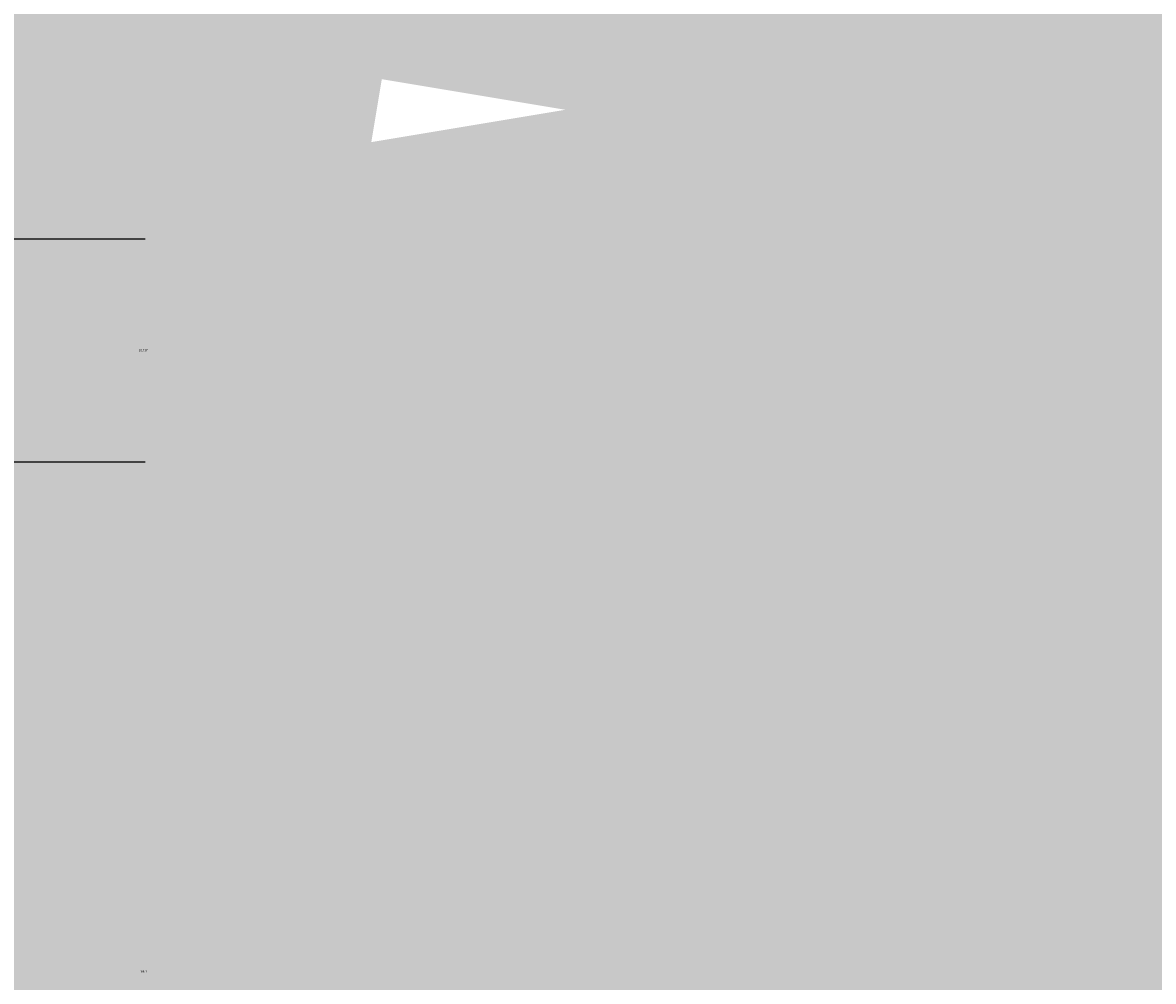
# Model space of a CAD drawing. Units: millimetres. Extents: x -22994 to 29398, y -19990 to 20176.
# Tile 124 of 135: x 296 to 391, y 92 to 173. Entities that reach past the tile are written whole.
import ezdxf

# ---------------------------------------------------------------- set-up
doc = ezdxf.new("R2010")
doc.units = ezdxf.units.MM
doc.header["$MEASUREMENT"] = 0
doc.layers.add('M-DIMS', color=2, linetype='Continuous', lineweight=18)
doc.styles.get("Standard").update_dxf_attribs({"font": 'arial.ttf'})
doc.dimstyles.get("Standard").update_dxf_attribs({"dimtxt": 0.18, "dimasz": 10000, "dimexe": 0.18, "dimexo": 0.0625, "dimgap": 0.09, "dimtad": 0, "dimtih": 1, "dimtoh": 1, "dimdec": 0, "dimzin": 0, "dimdsep": 46, "dimtxsty": 'Standard', "dimcen": 0.09, "dimadec": 0, "dimazin": 0, "dimtfac": 1, "dimtdec": 0, "dimtofl": 0, "dimtmove": 0, "dimatfit": 3, "dimfxl": 1, "dimtolj": 1, "dimtzin": 0, "dimlwd": 30, "dimarcsym": 0})

# ---------------------------------------------------------------- blocks, each defined once
blk = doc.blocks.new('*D2')
at = {"layer": 'Defpoints', "color": 0, "transparency": 16777216}
for p in [(6.677, 10.271), (290.852, 10.271), (290.852, -5.079)]:
    blk.add_point(p, dxfattribs=at)
at = {"layer": 'M-DIMS', "color": 0, "lineweight": -2, "transparency": 16777216}
for p, q in [((6.677, 10.209), (6.677, -5.259)), ((290.852, 10.209), (290.852, -5.259))]:
    blk.add_line(p, q, dxfattribs=at)
at = {"layer": 'M-DIMS', "color": 0, "lineweight": 30, "transparency": 16777216}
for p, q in [((-9993.323, -5.079), (-19993.323, -5.079)), ((10290.852, -5.079), (20290.852, -5.079))]:
    blk.add_line(p, q, dxfattribs=at)
at = {"layer": 'M-DIMS', "color": 0, "transparency": 16777216}
for points in [[(-9993.323, 1661.588), (-9993.323, -1671.745), (6.677, -5.079)], [(10290.852, 1661.588), (10290.852, -1671.745), (290.852, -5.079)]]:
    blk.add_solid(points, dxfattribs=at)
at = {"layer": 'M-DIMS', "color": 0, "transparency": 16777216, "insert": (148.765, -5.079), "char_height": 0.18, "attachment_point": 5}
blk.add_mtext('\\A1;284.2', dxfattribs=at)
blk = doc.blocks.new('*D3')
at = {"layer": 'Defpoints', "color": 0, "transparency": 16777216}
for p in [(110.265, 204.165), (110.265, 176.366), (95.833, 127.967)]:
    blk.add_point(p, dxfattribs=at)
at = {"layer": 'M-DIMS', "color": 0, "lineweight": 30, "transparency": 16777216}
for p, q in [((-9904.167, 204.165), (-19904.167, 204.165)), ((10110.265, 204.165), (20110.265, 204.165))]:
    blk.add_line(p, q, dxfattribs=at)
at = {"layer": 'M-DIMS', "color": 0, "lineweight": -2, "transparency": 16777216}
for p, q in [((95.833, 128.03), (95.833, 204.345)), ((110.265, 176.429), (110.265, 204.345))]:
    blk.add_line(p, q, dxfattribs=at)
at = {"layer": 'M-DIMS', "color": 0, "transparency": 16777216}
for points in [[(-9904.167, 1870.832), (-9904.167, -1462.501), (95.833, 204.165)], [(10110.265, 1870.832), (10110.265, -1462.501), (110.265, 204.165)]]:
    blk.add_solid(points, dxfattribs=at)
at = {"layer": 'M-DIMS', "color": 0, "transparency": 16777216, "insert": (103.049, 204.165), "char_height": 0.18, "attachment_point": 5}
blk.add_mtext('\\A1;14.432', dxfattribs=at)
blk = doc.blocks.new('*D4')
at = {"layer": 'Defpoints', "color": 0, "transparency": 16777216}
for p in [(116.265, 204.165), (110.265, 176.366), (116.265, 176.366)]:
    blk.add_point(p, dxfattribs=at)
at = {"layer": 'M-DIMS', "color": 0, "lineweight": 30, "transparency": 16777216}
for p, q in [((-9889.735, 204.165), (-19889.735, 204.165)), ((10116.265, 204.165), (20116.265, 204.165))]:
    blk.add_line(p, q, dxfattribs=at)
at = {"layer": 'M-DIMS', "color": 0, "lineweight": -2, "transparency": 16777216}
for p, q in [((110.265, 176.429), (110.265, 204.345)), ((116.265, 176.429), (116.265, 204.345))]:
    blk.add_line(p, q, dxfattribs=at)
at = {"layer": 'M-DIMS', "color": 0, "transparency": 16777216}
for points in [[(-9889.735, 1870.832), (-9889.735, -1462.501), (110.265, 204.165)], [(10116.265, 1870.832), (10116.265, -1462.501), (116.265, 204.165)]]:
    blk.add_solid(points, dxfattribs=at)
at = {"layer": 'M-DIMS', "color": 0, "transparency": 16777216, "insert": (113.265, 204.165), "char_height": 0.18, "attachment_point": 5}
blk.add_mtext('\\A1;6', dxfattribs=at)
blk = doc.blocks.new('*D5')
at = {"layer": 'Defpoints', "color": 0, "transparency": 16777216}
for p in [(181.265, 204.165), (116.265, 176.366), (181.265, 176.366)]:
    blk.add_point(p, dxfattribs=at)
at = {"layer": 'M-DIMS', "color": 0, "lineweight": 30, "transparency": 16777216}
for p, q in [((-9883.735, 204.165), (-19883.735, 204.165)), ((10181.265, 204.165), (20181.265, 204.165))]:
    blk.add_line(p, q, dxfattribs=at)
at = {"layer": 'M-DIMS', "color": 0, "lineweight": -2, "transparency": 16777216}
for p, q in [((116.265, 176.429), (116.265, 204.345)), ((181.265, 176.429), (181.265, 204.345))]:
    blk.add_line(p, q, dxfattribs=at)
at = {"layer": 'M-DIMS', "color": 0, "transparency": 16777216}
for points in [[(-9883.735, 1870.832), (-9883.735, -1462.501), (116.265, 204.165)], [(10181.265, 1870.832), (10181.265, -1462.501), (181.265, 204.165)]]:
    blk.add_solid(points, dxfattribs=at)
at = {"layer": 'M-DIMS', "color": 0, "transparency": 16777216, "insert": (148.765, 204.165), "char_height": 0.18, "attachment_point": 5}
blk.add_mtext('\\A1;65', dxfattribs=at)
blk = doc.blocks.new('*D6')
at = {"layer": 'Defpoints', "color": 0, "transparency": 16777216}
for p in [(187.265, 204.165), (181.265, 176.366), (187.265, 176.366)]:
    blk.add_point(p, dxfattribs=at)
at = {"layer": 'M-DIMS', "color": 0, "lineweight": 30, "transparency": 16777216}
for p, q in [((-9818.735, 204.165), (-19818.735, 204.165)), ((10187.265, 204.165), (20187.265, 204.165))]:
    blk.add_line(p, q, dxfattribs=at)
at = {"layer": 'M-DIMS', "color": 0, "lineweight": -2, "transparency": 16777216}
for p, q in [((181.265, 176.429), (181.265, 204.345)), ((187.265, 176.429), (187.265, 204.345))]:
    blk.add_line(p, q, dxfattribs=at)
at = {"layer": 'M-DIMS', "color": 0, "transparency": 16777216}
for points in [[(-9818.735, 1870.832), (-9818.735, -1462.501), (181.265, 204.165)], [(10187.265, 1870.832), (10187.265, -1462.501), (187.265, 204.165)]]:
    blk.add_solid(points, dxfattribs=at)
at = {"layer": 'M-DIMS', "color": 0, "transparency": 16777216, "insert": (184.265, 204.165), "char_height": 0.18, "attachment_point": 5}
blk.add_mtext('\\A1;6', dxfattribs=at)
blk = doc.blocks.new('*D7')
at = {"layer": 'Defpoints', "color": 0, "transparency": 16777216}
for p in [(201.697, 204.165), (187.265, 176.366), (201.697, 127.967)]:
    blk.add_point(p, dxfattribs=at)
at = {"layer": 'M-DIMS', "color": 0, "lineweight": 30, "transparency": 16777216}
for p, q in [((-9812.735, 204.165), (-19812.735, 204.165)), ((10201.697, 204.165), (20201.697, 204.165))]:
    blk.add_line(p, q, dxfattribs=at)
at = {"layer": 'M-DIMS', "color": 0, "lineweight": -2, "transparency": 16777216}
for p, q in [((187.265, 176.429), (187.265, 204.345)), ((201.697, 128.03), (201.697, 204.345))]:
    blk.add_line(p, q, dxfattribs=at)
at = {"layer": 'M-DIMS', "color": 0, "transparency": 16777216}
for points in [[(-9812.735, 1870.832), (-9812.735, -1462.501), (187.265, 204.165)], [(10201.697, 1870.832), (10201.697, -1462.501), (201.697, 204.165)]]:
    blk.add_solid(points, dxfattribs=at)
at = {"layer": 'M-DIMS', "color": 0, "transparency": 16777216, "insert": (194.481, 204.165), "char_height": 0.18, "attachment_point": 5}
blk.add_mtext('\\A1;14.432', dxfattribs=at)
blk = doc.blocks.new('*D8')
at = {"layer": 'Defpoints', "color": 0, "transparency": 16777216}
for p in [(227.648, 204.165), (227.648, 146.73), (201.697, 127.967)]:
    blk.add_point(p, dxfattribs=at)
at = {"layer": 'M-DIMS', "color": 0, "lineweight": 30, "transparency": 16777216}
for p, q in [((-9798.303, 204.165), (-19798.303, 204.165)), ((10227.648, 204.165), (20227.648, 204.165))]:
    blk.add_line(p, q, dxfattribs=at)
at = {"layer": 'M-DIMS', "color": 0, "lineweight": -2, "transparency": 16777216}
for p, q in [((201.697, 128.03), (201.697, 204.345)), ((227.648, 146.792), (227.648, 204.345))]:
    blk.add_line(p, q, dxfattribs=at)
at = {"layer": 'M-DIMS', "color": 0, "transparency": 16777216}
for points in [[(-9798.303, 1870.832), (-9798.303, -1462.501), (201.697, 204.165)], [(10227.648, 1870.832), (10227.648, -1462.501), (227.648, 204.165)]]:
    blk.add_solid(points, dxfattribs=at)
at = {"layer": 'M-DIMS', "color": 0, "transparency": 16777216, "insert": (214.673, 204.165), "char_height": 0.18, "attachment_point": 5}
blk.add_mtext('\\A1;25.95', dxfattribs=at)
blk = doc.blocks.new('*D9')
at = {"layer": 'Defpoints', "color": 0, "transparency": 16777216}
for p in [(187.265, 176.366), (306.202, 176.366), (290.852, 10.271)]:
    blk.add_point(p, dxfattribs=at)
at = {"layer": 'M-DIMS', "color": 0, "lineweight": 30, "transparency": 16777216}
for p, q in [((306.202, 10176.366), (306.202, 20176.366)), ((306.202, -9989.729), (306.202, -19989.729))]:
    blk.add_line(p, q, dxfattribs=at)
at = {"layer": 'M-DIMS', "color": 0, "lineweight": -2, "transparency": 16777216}
for p, q in [((187.327, 176.366), (306.382, 176.366)), ((290.915, 10.271), (306.382, 10.271))]:
    blk.add_line(p, q, dxfattribs=at)
at = {"layer": 'M-DIMS', "color": 0, "transparency": 16777216}
for points in [[(-1360.465, 10176.366), (1972.869, 10176.366), (306.202, 176.366)], [(-1360.465, -9989.729), (1972.869, -9989.729), (306.202, 10.271)]]:
    blk.add_solid(points, dxfattribs=at)
at = {"layer": 'M-DIMS', "color": 0, "transparency": 16777216, "insert": (306.202, 93.319), "char_height": 0.18, "attachment_point": 5}
blk.add_mtext('\\A1;166.1', dxfattribs=at)
blk = doc.blocks.new('*D10')
at = {"layer": 'Defpoints', "color": 0, "transparency": 16777216}
for p in [(125.65, 136.071), (133.346, 136.071), (133.346, -5.079)]:
    blk.add_point(p, dxfattribs=at)
at = {"layer": 'M-DIMS', "color": 0, "lineweight": -2, "transparency": 16777216}
for p, q in [((125.65, 136.009), (125.65, -5.259)), ((133.346, 136.009), (133.346, -5.259))]:
    blk.add_line(p, q, dxfattribs=at)
at = {"layer": 'M-DIMS', "color": 0, "lineweight": 30, "transparency": 16777216}
for p, q in [((-9874.35, -5.079), (-19874.35, -5.079)), ((10133.346, -5.079), (20133.346, -5.079))]:
    blk.add_line(p, q, dxfattribs=at)
at = {"layer": 'M-DIMS', "color": 0, "transparency": 16777216}
for points in [[(-9874.35, 1661.588), (-9874.35, -1671.745), (125.65, -5.079)], [(10133.346, 1661.588), (10133.346, -1671.745), (133.346, -5.079)]]:
    blk.add_solid(points, dxfattribs=at)
at = {"layer": 'M-DIMS', "color": 0, "transparency": 16777216, "insert": (129.498, -5.079), "char_height": 0.18, "attachment_point": 5}
blk.add_mtext('\\A1;7.696', dxfattribs=at)
blk = doc.blocks.new('*D11')
at = {"layer": 'Defpoints', "color": 0, "transparency": 16777216}
for p in [(133.346, 136.071), (135.65, 136.071), (135.65, -5.079)]:
    blk.add_point(p, dxfattribs=at)
at = {"layer": 'M-DIMS', "color": 0, "lineweight": -2, "transparency": 16777216}
for p, q in [((133.346, 136.009), (133.346, -5.259)), ((135.65, 136.009), (135.65, -5.259))]:
    blk.add_line(p, q, dxfattribs=at)
at = {"layer": 'M-DIMS', "color": 0, "lineweight": 30, "transparency": 16777216}
for p, q in [((-9866.654, -5.079), (-19866.654, -5.079)), ((10135.65, -5.079), (20135.65, -5.079))]:
    blk.add_line(p, q, dxfattribs=at)
at = {"layer": 'M-DIMS', "color": 0, "transparency": 16777216}
for points in [[(-9866.654, 1661.588), (-9866.654, -1671.745), (133.346, -5.079)], [(10135.65, 1661.588), (10135.65, -1671.745), (135.65, -5.079)]]:
    blk.add_solid(points, dxfattribs=at)
at = {"layer": 'M-DIMS', "color": 0, "transparency": 16777216, "insert": (134.498, -5.079), "char_height": 0.18, "attachment_point": 5}
blk.add_mtext('\\A1;2.304', dxfattribs=at)
blk = doc.blocks.new('*D12')
at = {"layer": 'Defpoints', "color": 0, "transparency": 16777216}
for p in [(135.65, 136.071), (145.65, 136.071), (145.65, -5.079)]:
    blk.add_point(p, dxfattribs=at)
at = {"layer": 'M-DIMS', "color": 0, "lineweight": -2, "transparency": 16777216}
for p, q in [((135.65, 136.009), (135.65, -5.259)), ((145.65, 136.009), (145.65, -5.259))]:
    blk.add_line(p, q, dxfattribs=at)
at = {"layer": 'M-DIMS', "color": 0, "lineweight": 30, "transparency": 16777216}
for p, q in [((-9864.35, -5.079), (-19864.35, -5.079)), ((10145.65, -5.079), (20145.65, -5.079))]:
    blk.add_line(p, q, dxfattribs=at)
at = {"layer": 'M-DIMS', "color": 0, "transparency": 16777216}
for points in [[(-9864.35, 1661.588), (-9864.35, -1671.745), (135.65, -5.079)], [(10145.65, 1661.588), (10145.65, -1671.745), (145.65, -5.079)]]:
    blk.add_solid(points, dxfattribs=at)
at = {"layer": 'M-DIMS', "color": 0, "transparency": 16777216, "insert": (140.65, -5.079), "char_height": 0.18, "attachment_point": 5}
blk.add_mtext('\\A1;10', dxfattribs=at)
blk = doc.blocks.new('*D13')
at = {"layer": 'Defpoints', "color": 0, "transparency": 16777216}
for p in [(145.65, 136.071), (155.65, 136.071), (155.65, -5.079)]:
    blk.add_point(p, dxfattribs=at)
at = {"layer": 'M-DIMS', "color": 0, "lineweight": -2, "transparency": 16777216}
for p, q in [((145.65, 136.009), (145.65, -5.259)), ((155.65, 136.009), (155.65, -5.259))]:
    blk.add_line(p, q, dxfattribs=at)
at = {"layer": 'M-DIMS', "color": 0, "lineweight": 30, "transparency": 16777216}
for p, q in [((-9854.35, -5.079), (-19854.35, -5.079)), ((10155.65, -5.079), (20155.65, -5.079))]:
    blk.add_line(p, q, dxfattribs=at)
at = {"layer": 'M-DIMS', "color": 0, "transparency": 16777216}
for points in [[(-9854.35, 1661.588), (-9854.35, -1671.745), (145.65, -5.079)], [(10155.65, 1661.588), (10155.65, -1671.745), (155.65, -5.079)]]:
    blk.add_solid(points, dxfattribs=at)
at = {"layer": 'M-DIMS', "color": 0, "transparency": 16777216, "insert": (150.65, -5.079), "char_height": 0.18, "attachment_point": 5}
blk.add_mtext('\\A1;10', dxfattribs=at)
blk = doc.blocks.new('*D14')
at = {"layer": 'Defpoints', "color": 0, "transparency": 16777216}
for p in [(155.65, 136.071), (165.65, 136.071), (165.65, -5.079)]:
    blk.add_point(p, dxfattribs=at)
at = {"layer": 'M-DIMS', "color": 0, "lineweight": -2, "transparency": 16777216}
for p, q in [((155.65, 136.009), (155.65, -5.259)), ((165.65, 136.009), (165.65, -5.259))]:
    blk.add_line(p, q, dxfattribs=at)
at = {"layer": 'M-DIMS', "color": 0, "lineweight": 30, "transparency": 16777216}
for p, q in [((-9844.35, -5.079), (-19844.35, -5.079)), ((10165.65, -5.079), (20165.65, -5.079))]:
    blk.add_line(p, q, dxfattribs=at)
at = {"layer": 'M-DIMS', "color": 0, "transparency": 16777216}
for points in [[(-9844.35, 1661.588), (-9844.35, -1671.745), (155.65, -5.079)], [(10165.65, 1661.588), (10165.65, -1671.745), (165.65, -5.079)]]:
    blk.add_solid(points, dxfattribs=at)
at = {"layer": 'M-DIMS', "color": 0, "transparency": 16777216, "insert": (160.65, -5.079), "char_height": 0.18, "attachment_point": 5}
blk.add_mtext('\\A1;10', dxfattribs=at)
blk = doc.blocks.new('*D15')
at = {"layer": 'Defpoints', "color": 0, "transparency": 16777216}
for p in [(173.346, 154.788), (173.346, 136.071), (306.202, 136.071)]:
    blk.add_point(p, dxfattribs=at)
at = {"layer": 'M-DIMS', "color": 0, "lineweight": 30, "transparency": 16777216}
for p, q in [((306.202, 10154.788), (306.202, 20154.788)), ((306.202, -9863.929), (306.202, -19863.929))]:
    blk.add_line(p, q, dxfattribs=at)
at = {"layer": 'M-DIMS', "color": 0, "lineweight": -2, "transparency": 16777216}
for p, q in [((173.408, 154.788), (306.382, 154.788)), ((173.408, 136.071), (306.382, 136.071))]:
    blk.add_line(p, q, dxfattribs=at)
at = {"layer": 'M-DIMS', "color": 0, "transparency": 16777216}
for points in [[(-1360.465, 10154.788), (1972.869, 10154.788), (306.202, 154.788)], [(-1360.465, -9863.929), (1972.869, -9863.929), (306.202, 136.071)]]:
    blk.add_solid(points, dxfattribs=at)
at = {"layer": 'M-DIMS', "color": 0, "transparency": 16777216, "insert": (306.202, 145.43), "char_height": 0.18, "attachment_point": 5}
blk.add_mtext('\\A1;18.717', dxfattribs=at)
blk = doc.blocks.new('*D16')
at = {"layer": 'Defpoints', "color": 0, "transparency": 16777216}
for p in [(120.17, 204.165), (110.466, 48.035), (120.17, 48.035)]:
    blk.add_point(p, dxfattribs=at)
at = {"layer": 'M-DIMS', "color": 0, "lineweight": 30, "transparency": 16777216}
for p, q in [((-9889.534, 204.165), (-19889.534, 204.165)), ((10120.17, 204.165), (20120.17, 204.165))]:
    blk.add_line(p, q, dxfattribs=at)
at = {"layer": 'M-DIMS', "color": 0, "lineweight": -2, "transparency": 16777216}
for p, q in [((110.466, 48.097), (110.466, 204.345)), ((120.17, 48.097), (120.17, 204.345))]:
    blk.add_line(p, q, dxfattribs=at)
at = {"layer": 'M-DIMS', "color": 0, "transparency": 16777216}
for points in [[(-9889.534, 1870.832), (-9889.534, -1462.501), (110.466, 204.165)], [(10120.17, 1870.832), (10120.17, -1462.501), (120.17, 204.165)]]:
    blk.add_solid(points, dxfattribs=at)
at = {"layer": 'M-DIMS', "color": 0, "transparency": 16777216, "insert": (115.318, 204.165), "char_height": 0.18, "attachment_point": 5}
blk.add_mtext('\\A1;9.704', dxfattribs=at)
blk = doc.blocks.new('*D17')
at = {"layer": 'Defpoints', "color": 0, "transparency": 16777216}
for p in [(126.17, 204.165), (120.17, 48.035), (126.17, 48.035)]:
    blk.add_point(p, dxfattribs=at)
at = {"layer": 'M-DIMS', "color": 0, "lineweight": 30, "transparency": 16777216}
for p, q in [((-9879.83, 204.165), (-19879.83, 204.165)), ((10126.17, 204.165), (20126.17, 204.165))]:
    blk.add_line(p, q, dxfattribs=at)
at = {"layer": 'M-DIMS', "color": 0, "lineweight": -2, "transparency": 16777216}
for p, q in [((120.17, 48.097), (120.17, 204.345)), ((126.17, 48.097), (126.17, 204.345))]:
    blk.add_line(p, q, dxfattribs=at)
at = {"layer": 'M-DIMS', "color": 0, "transparency": 16777216}
for points in [[(-9879.83, 1870.832), (-9879.83, -1462.501), (120.17, 204.165)], [(10126.17, 1870.832), (10126.17, -1462.501), (126.17, 204.165)]]:
    blk.add_solid(points, dxfattribs=at)
at = {"layer": 'M-DIMS', "color": 0, "transparency": 16777216, "insert": (123.17, 204.165), "char_height": 0.18, "attachment_point": 5}
blk.add_mtext('\\A1;6', dxfattribs=at)
blk = doc.blocks.new('*D18')
at = {"layer": 'Defpoints', "color": 0, "transparency": 16777216}
for p in [(132.17, 204.165), (126.17, 48.035), (132.17, 48.035)]:
    blk.add_point(p, dxfattribs=at)
at = {"layer": 'M-DIMS', "color": 0, "lineweight": 30, "transparency": 16777216}
for p, q in [((-9873.83, 204.165), (-19873.83, 204.165)), ((10132.17, 204.165), (20132.17, 204.165))]:
    blk.add_line(p, q, dxfattribs=at)
at = {"layer": 'M-DIMS', "color": 0, "lineweight": -2, "transparency": 16777216}
for p, q in [((126.17, 48.097), (126.17, 204.345)), ((132.17, 48.097), (132.17, 204.345))]:
    blk.add_line(p, q, dxfattribs=at)
at = {"layer": 'M-DIMS', "color": 0, "transparency": 16777216}
for points in [[(-9873.83, 1870.832), (-9873.83, -1462.501), (126.17, 204.165)], [(10132.17, 1870.832), (10132.17, -1462.501), (132.17, 204.165)]]:
    blk.add_solid(points, dxfattribs=at)
at = {"layer": 'M-DIMS', "color": 0, "transparency": 16777216, "insert": (129.17, 204.165), "char_height": 0.18, "attachment_point": 5}
blk.add_mtext('\\A1;6', dxfattribs=at)
blk = doc.blocks.new('*D19')
at = {"layer": 'Defpoints', "color": 0, "transparency": 16777216}
for p in [(138.17, 204.165), (132.17, 48.035), (138.17, 48.035)]:
    blk.add_point(p, dxfattribs=at)
at = {"layer": 'M-DIMS', "color": 0, "lineweight": 30, "transparency": 16777216}
for p, q in [((-9867.83, 204.165), (-19867.83, 204.165)), ((10138.17, 204.165), (20138.17, 204.165))]:
    blk.add_line(p, q, dxfattribs=at)
at = {"layer": 'M-DIMS', "color": 0, "lineweight": -2, "transparency": 16777216}
for p, q in [((132.17, 48.097), (132.17, 204.345)), ((138.17, 48.097), (138.17, 204.345))]:
    blk.add_line(p, q, dxfattribs=at)
at = {"layer": 'M-DIMS', "color": 0, "transparency": 16777216}
for points in [[(-9867.83, 1870.832), (-9867.83, -1462.501), (132.17, 204.165)], [(10138.17, 1870.832), (10138.17, -1462.501), (138.17, 204.165)]]:
    blk.add_solid(points, dxfattribs=at)
at = {"layer": 'M-DIMS', "color": 0, "transparency": 16777216, "insert": (135.17, 204.165), "char_height": 0.18, "attachment_point": 5}
blk.add_mtext('\\A1;6', dxfattribs=at)
blk = doc.blocks.new('*D20')
at = {"layer": 'Defpoints', "color": 0, "transparency": 16777216}
for p in [(144.17, 204.165), (138.17, 48.035), (144.17, 48.035)]:
    blk.add_point(p, dxfattribs=at)
at = {"layer": 'M-DIMS', "color": 0, "lineweight": 30, "transparency": 16777216}
for p, q in [((-9861.83, 204.165), (-19861.83, 204.165)), ((10144.17, 204.165), (20144.17, 204.165))]:
    blk.add_line(p, q, dxfattribs=at)
at = {"layer": 'M-DIMS', "color": 0, "lineweight": -2, "transparency": 16777216}
for p, q in [((138.17, 48.097), (138.17, 204.345)), ((144.17, 48.097), (144.17, 204.345))]:
    blk.add_line(p, q, dxfattribs=at)
at = {"layer": 'M-DIMS', "color": 0, "transparency": 16777216}
for points in [[(-9861.83, 1870.832), (-9861.83, -1462.501), (138.17, 204.165)], [(10144.17, 1870.832), (10144.17, -1462.501), (144.17, 204.165)]]:
    blk.add_solid(points, dxfattribs=at)
at = {"layer": 'M-DIMS', "color": 0, "transparency": 16777216, "insert": (141.17, 204.165), "char_height": 0.18, "attachment_point": 5}
blk.add_mtext('\\A1;6', dxfattribs=at)
blk = doc.blocks.new('*D21')
at = {"layer": 'Defpoints', "color": 0, "transparency": 16777216}
for p in [(149.116, 204.165), (144.17, 48.035), (149.116, 48.035)]:
    blk.add_point(p, dxfattribs=at)
at = {"layer": 'M-DIMS', "color": 0, "lineweight": 30, "transparency": 16777216}
for p, q in [((-9855.83, 204.165), (-19855.83, 204.165)), ((10149.116, 204.165), (20149.116, 204.165))]:
    blk.add_line(p, q, dxfattribs=at)
at = {"layer": 'M-DIMS', "color": 0, "lineweight": -2, "transparency": 16777216}
for p, q in [((144.17, 48.097), (144.17, 204.345)), ((149.116, 48.097), (149.116, 204.345))]:
    blk.add_line(p, q, dxfattribs=at)
at = {"layer": 'M-DIMS', "color": 0, "transparency": 16777216}
for points in [[(-9855.83, 1870.832), (-9855.83, -1462.501), (144.17, 204.165)], [(10149.116, 1870.832), (10149.116, -1462.501), (149.116, 204.165)]]:
    blk.add_solid(points, dxfattribs=at)
at = {"layer": 'M-DIMS', "color": 0, "transparency": 16777216, "insert": (146.643, 204.165), "char_height": 0.18, "attachment_point": 5}
blk.add_mtext('\\A1;4.945', dxfattribs=at)
blk = doc.blocks.new('*D22')
at = {"layer": 'Defpoints', "color": 0, "transparency": 16777216}
for p in [(149.116, 30.99), (155.116, 30.99), (155.116, -5.079)]:
    blk.add_point(p, dxfattribs=at)
at = {"layer": 'M-DIMS', "color": 0, "lineweight": -2, "transparency": 16777216}
for p, q in [((149.116, 30.927), (149.116, -5.259)), ((155.116, 30.927), (155.116, -5.259))]:
    blk.add_line(p, q, dxfattribs=at)
at = {"layer": 'M-DIMS', "color": 0, "lineweight": 30, "transparency": 16777216}
for p, q in [((-9850.884, -5.079), (-19850.884, -5.079)), ((10155.116, -5.079), (20155.116, -5.079))]:
    blk.add_line(p, q, dxfattribs=at)
at = {"layer": 'M-DIMS', "color": 0, "transparency": 16777216}
for points in [[(-9850.884, 1661.588), (-9850.884, -1671.745), (149.116, -5.079)], [(10155.116, 1661.588), (10155.116, -1671.745), (155.116, -5.079)]]:
    blk.add_solid(points, dxfattribs=at)
at = {"layer": 'M-DIMS', "color": 0, "transparency": 16777216, "insert": (152.116, -5.079), "char_height": 0.18, "attachment_point": 5}
blk.add_mtext('\\A1;6', dxfattribs=at)
blk = doc.blocks.new('*D23')
at = {"layer": 'Defpoints', "color": 0, "transparency": 16777216}
for p in [(155.116, 30.99), (161.116, 30.99), (161.116, -5.079)]:
    blk.add_point(p, dxfattribs=at)
at = {"layer": 'M-DIMS', "color": 0, "lineweight": -2, "transparency": 16777216}
for p, q in [((155.116, 30.927), (155.116, -5.259)), ((161.116, 30.927), (161.116, -5.259))]:
    blk.add_line(p, q, dxfattribs=at)
at = {"layer": 'M-DIMS', "color": 0, "lineweight": 30, "transparency": 16777216}
for p, q in [((-9844.884, -5.079), (-19844.884, -5.079)), ((10161.116, -5.079), (20161.116, -5.079))]:
    blk.add_line(p, q, dxfattribs=at)
at = {"layer": 'M-DIMS', "color": 0, "transparency": 16777216}
for points in [[(-9844.884, 1661.588), (-9844.884, -1671.745), (155.116, -5.079)], [(10161.116, 1661.588), (10161.116, -1671.745), (161.116, -5.079)]]:
    blk.add_solid(points, dxfattribs=at)
at = {"layer": 'M-DIMS', "color": 0, "transparency": 16777216, "insert": (158.116, -5.079), "char_height": 0.18, "attachment_point": 5}
blk.add_mtext('\\A1;6', dxfattribs=at)
blk = doc.blocks.new('*D24')
at = {"layer": 'Defpoints', "color": 0, "transparency": 16777216}
for p in [(161.116, 30.99), (166.439, 30.99), (166.439, -5.079)]:
    blk.add_point(p, dxfattribs=at)
at = {"layer": 'M-DIMS', "color": 0, "lineweight": -2, "transparency": 16777216}
for p, q in [((161.116, 30.927), (161.116, -5.259)), ((166.439, 30.927), (166.439, -5.259))]:
    blk.add_line(p, q, dxfattribs=at)
at = {"layer": 'M-DIMS', "color": 0, "lineweight": 30, "transparency": 16777216}
for p, q in [((-9838.884, -5.079), (-19838.884, -5.079)), ((10166.439, -5.079), (20166.439, -5.079))]:
    blk.add_line(p, q, dxfattribs=at)
at = {"layer": 'M-DIMS', "color": 0, "transparency": 16777216}
for points in [[(-9838.884, 1661.588), (-9838.884, -1671.745), (161.116, -5.079)], [(10166.439, 1661.588), (10166.439, -1671.745), (166.439, -5.079)]]:
    blk.add_solid(points, dxfattribs=at)
at = {"layer": 'M-DIMS', "color": 0, "transparency": 16777216, "insert": (163.777, -5.079), "char_height": 0.18, "attachment_point": 5}
blk.add_mtext('\\A1;5.323', dxfattribs=at)
blk = doc.blocks.new('*D25')
at = {"layer": 'Defpoints', "color": 0, "transparency": 16777216}
for p in [(166.439, 30.99), (172.439, 30.99), (172.439, -5.079)]:
    blk.add_point(p, dxfattribs=at)
at = {"layer": 'M-DIMS', "color": 0, "lineweight": -2, "transparency": 16777216}
for p, q in [((166.439, 30.927), (166.439, -5.259)), ((172.439, 30.927), (172.439, -5.259))]:
    blk.add_line(p, q, dxfattribs=at)
at = {"layer": 'M-DIMS', "color": 0, "lineweight": 30, "transparency": 16777216}
for p, q in [((-9833.561, -5.079), (-19833.561, -5.079)), ((10172.439, -5.079), (20172.439, -5.079))]:
    blk.add_line(p, q, dxfattribs=at)
at = {"layer": 'M-DIMS', "color": 0, "transparency": 16777216}
for points in [[(-9833.561, 1661.588), (-9833.561, -1671.745), (166.439, -5.079)], [(10172.439, 1661.588), (10172.439, -1671.745), (172.439, -5.079)]]:
    blk.add_solid(points, dxfattribs=at)
at = {"layer": 'M-DIMS', "color": 0, "transparency": 16777216, "insert": (169.439, -5.079), "char_height": 0.18, "attachment_point": 5}
blk.add_mtext('\\A1;6', dxfattribs=at)
blk = doc.blocks.new('*D26')
at = {"layer": 'Defpoints', "color": 0, "transparency": 16777216}
for p in [(172.439, 30.99), (178.439, 30.99), (178.439, -5.079)]:
    blk.add_point(p, dxfattribs=at)
at = {"layer": 'M-DIMS', "color": 0, "lineweight": -2, "transparency": 16777216}
for p, q in [((172.439, 30.927), (172.439, -5.259)), ((178.439, 30.927), (178.439, -5.259))]:
    blk.add_line(p, q, dxfattribs=at)
at = {"layer": 'M-DIMS', "color": 0, "lineweight": 30, "transparency": 16777216}
for p, q in [((-9827.561, -5.079), (-19827.561, -5.079)), ((10178.439, -5.079), (20178.439, -5.079))]:
    blk.add_line(p, q, dxfattribs=at)
at = {"layer": 'M-DIMS', "color": 0, "transparency": 16777216}
for points in [[(-9827.561, 1661.588), (-9827.561, -1671.745), (172.439, -5.079)], [(10178.439, 1661.588), (10178.439, -1671.745), (178.439, -5.079)]]:
    blk.add_solid(points, dxfattribs=at)
at = {"layer": 'M-DIMS', "color": 0, "transparency": 16777216, "insert": (175.439, -5.079), "char_height": 0.18, "attachment_point": 5}
blk.add_mtext('\\A1;6', dxfattribs=at)
blk = doc.blocks.new('*D27')
at = {"layer": 'Defpoints', "color": 0, "transparency": 16777216}
for p in [(178.439, 30.99), (188.117, 30.99), (188.117, -5.079)]:
    blk.add_point(p, dxfattribs=at)
at = {"layer": 'M-DIMS', "color": 0, "lineweight": -2, "transparency": 16777216}
for p, q in [((178.439, 30.927), (178.439, -5.259)), ((188.117, 30.927), (188.117, -5.259))]:
    blk.add_line(p, q, dxfattribs=at)
at = {"layer": 'M-DIMS', "color": 0, "lineweight": 30, "transparency": 16777216}
for p, q in [((-9821.561, -5.079), (-19821.561, -5.079)), ((10188.117, -5.079), (20188.117, -5.079))]:
    blk.add_line(p, q, dxfattribs=at)
at = {"layer": 'M-DIMS', "color": 0, "transparency": 16777216}
for points in [[(-9821.561, 1661.588), (-9821.561, -1671.745), (178.439, -5.079)], [(10188.117, 1661.588), (10188.117, -1671.745), (188.117, -5.079)]]:
    blk.add_solid(points, dxfattribs=at)
at = {"layer": 'M-DIMS', "color": 0, "transparency": 16777216, "insert": (183.278, -5.079), "char_height": 0.18, "attachment_point": 5}
blk.add_mtext('\\A1;9.679', dxfattribs=at)
blk = doc.blocks.new('*D28')
at = {"layer": 'Defpoints', "color": 0, "transparency": 16777216}
for p in [(188.117, 48.035), (306.202, 48.035), (188.117, 30.99)]:
    blk.add_point(p, dxfattribs=at)
at = {"layer": 'M-DIMS', "color": 0, "lineweight": 30, "transparency": 16777216}
for p, q in [((306.202, 10048.035), (306.202, 20048.035)), ((306.202, -9969.01), (306.202, -19969.01))]:
    blk.add_line(p, q, dxfattribs=at)
at = {"layer": 'M-DIMS', "color": 0, "lineweight": -2, "transparency": 16777216}
for p, q in [((188.18, 48.035), (306.382, 48.035)), ((188.18, 30.99), (306.382, 30.99))]:
    blk.add_line(p, q, dxfattribs=at)
at = {"layer": 'M-DIMS', "color": 0, "transparency": 16777216}
for points in [[(-1360.465, 10048.035), (1972.869, 10048.035), (306.202, 48.035)], [(-1360.465, -9969.01), (1972.869, -9969.01), (306.202, 30.99)]]:
    blk.add_solid(points, dxfattribs=at)
at = {"layer": 'M-DIMS', "color": 0, "transparency": 16777216, "insert": (306.202, 39.512), "char_height": 0.18, "attachment_point": 5}
blk.add_mtext('\\A1;17.045', dxfattribs=at)
blk = doc.blocks.new('*D29')
at = {"layer": 'Defpoints', "color": 0, "transparency": 16777216}
for p in [(36.801, 80.045), (64.03, 80.045)]:
    blk.add_point(p, dxfattribs=at)
at = {"layer": 'M-DIMS', "color": 0, "lineweight": -2, "transparency": 16777216}
for p, q in [((50.325, 80.045), (50.505, 80.045)), ((50.415, 79.955), (50.415, 80.135))]:
    blk.add_line(p, q, dxfattribs=at)
at = {"layer": 'M-DIMS', "color": 0, "lineweight": 30, "transparency": 16777216}
blk.add_line((20064.03, 80.03), (10064.03, 80.038), dxfattribs=at)
at = {"layer": 'M-DIMS', "color": 0, "transparency": 16777216}
blk.add_solid([(10064.031, 1746.704), (10064.028, -1586.629), (64.03, 80.045)], dxfattribs=at)
at = {"layer": 'M-DIMS', "color": 0, "transparency": 16777216, "insert": (20064.521, 80.03), "char_height": 0.18, "attachment_point": 5}
blk.add_mtext('\\A1;∅27.23', dxfattribs=at)
blk = doc.blocks.new('*D30')
at = {"layer": 'Defpoints', "color": 0, "transparency": 16777216}
for p in [(216.315, 146.729), (238.982, 146.73)]:
    blk.add_point(p, dxfattribs=at)
at = {"layer": 'M-DIMS', "color": 0, "lineweight": 30, "transparency": 16777216}
blk.add_line((20238.982, 147.496), (10238.982, 147.113), dxfattribs=at)
at = {"layer": 'M-DIMS', "color": 0, "lineweight": -2, "transparency": 16777216}
for p, q in [((227.558, 146.73), (227.738, 146.73)), ((227.648, 146.64), (227.648, 146.82))]:
    blk.add_line(p, q, dxfattribs=at)
at = {"layer": 'M-DIMS', "color": 0, "transparency": 16777216}
blk.add_solid([(10238.918, 1813.78), (10239.046, -1519.554), (238.982, 146.73)], dxfattribs=at)
at = {"layer": 'M-DIMS', "color": 0, "transparency": 16777216, "insert": (20239.544, 147.496), "char_height": 0.18, "attachment_point": 5}
blk.add_mtext('\\A1;∅22.667', dxfattribs=at)
blk = doc.blocks.new('*D31')
at = {"layer": 'Defpoints', "color": 0, "transparency": 16777216}
for p in [(223.164, 146.729), (232.133, 146.73)]:
    blk.add_point(p, dxfattribs=at)
at = {"layer": 'M-DIMS', "color": 0, "lineweight": 30, "transparency": 16777216}
blk.add_line((20232.133, 148.666), (10232.133, 147.698), dxfattribs=at)
at = {"layer": 'M-DIMS', "color": 0, "lineweight": -2, "transparency": 16777216}
for p, q in [((227.558, 146.73), (227.738, 146.73)), ((227.648, 146.64), (227.648, 146.82))]:
    blk.add_line(p, q, dxfattribs=at)
at = {"layer": 'M-DIMS', "color": 0, "transparency": 16777216}
blk.add_solid([(10231.971, 1814.364), (10232.294, -1518.969), (232.133, 146.73)], dxfattribs=at)
at = {"layer": 'M-DIMS', "color": 0, "transparency": 16777216, "insert": (20232.625, 148.666), "char_height": 0.18, "attachment_point": 5}
blk.add_mtext('\\A1;∅8.969', dxfattribs=at)
blk = doc.blocks.new('*D33')
at = {"layer": 'Defpoints', "color": 0, "transparency": 16777216}
for p in [(229.561, 154.377), (232.997, 153.351)]:
    blk.add_point(p, dxfattribs=at)
at = {"layer": 'M-DIMS', "color": 0, "lineweight": -2, "transparency": 16777216}
for p, q in [((229.471, 154.377), (229.651, 154.377)), ((229.561, 154.287), (229.561, 154.467))]:
    blk.add_line(p, q, dxfattribs=at)
at = {"layer": 'M-DIMS', "color": 0, "lineweight": 30, "transparency": 16777216}
for p, q in [((19396.339, -5570.838), (9814.668, -2708.743)), ((29396.339, -5570.838), (19396.339, -5570.838))]:
    blk.add_line(p, q, dxfattribs=at)
at = {"layer": 'M-DIMS', "color": 0, "transparency": 16777216}
blk.add_solid([(10291.684, -1111.798), (9337.652, -4305.689), (232.997, 153.351)], dxfattribs=at)
at = {"layer": 'M-DIMS', "color": 0, "transparency": 16777216, "insert": (29397.012, -5570.838), "char_height": 0.18, "attachment_point": 5}
blk.add_mtext('\\A1;6X R3.586', dxfattribs=at)
blk = doc.blocks.new('*D34')
at = {"layer": 'Defpoints', "color": 0, "transparency": 16777216}
for p in [(178.58, 122.895), (176.812, 121.128)]:
    blk.add_point(p, dxfattribs=at)
at = {"layer": 'M-DIMS', "color": 0, "lineweight": 30, "transparency": 16777216}
for p, q in [((14322.436, 14263.311), (7250.508, 7193.103)), ((24322.436, 14263.311), (14322.436, 14263.311))]:
    blk.add_line(p, q, dxfattribs=at)
at = {"layer": 'M-DIMS', "color": 0, "lineweight": -2, "transparency": 16777216}
for p, q in [((176.722, 121.128), (176.902, 121.128)), ((176.812, 121.038), (176.812, 121.218))]:
    blk.add_line(p, q, dxfattribs=at)
at = {"layer": 'M-DIMS', "color": 0, "transparency": 16777216}
blk.add_solid([(6072.14, 8371.758), (8428.876, 6014.448), (178.58, 122.895)], dxfattribs=at)
at = {"layer": 'M-DIMS', "color": 0, "transparency": 16777216, "insert": (24322.97, 14263.311), "char_height": 0.18, "attachment_point": 5}
blk.add_mtext('\\A1;6X R2.5', dxfattribs=at)
blk = doc.blocks.new('*D36')
at = {"layer": 'Defpoints', "color": 0, "transparency": 16777216}
for p in [(46.39, 31.303), (46.387, 26.593)]:
    blk.add_point(p, dxfattribs=at)
at = {"layer": 'M-DIMS', "color": 0, "lineweight": 30, "transparency": 16777216}
for p, q in [((57.15, 20031.301), (51.77, 10031.302)), ((10057.15, 20031.301), (57.15, 20031.301))]:
    blk.add_line(p, q, dxfattribs=at)
at = {"layer": 'M-DIMS', "color": 0, "lineweight": -2, "transparency": 16777216}
for p, q in [((46.299, 28.948), (46.479, 28.948)), ((46.389, 28.858), (46.389, 29.038))]:
    blk.add_line(p, q, dxfattribs=at)
at = {"layer": 'M-DIMS', "color": 0, "transparency": 16777216}
blk.add_solid([(-1614.896, 10032.199), (1718.436, 10030.405), (46.39, 31.303)], dxfattribs=at)
at = {"layer": 'M-DIMS', "color": 0, "transparency": 16777216, "insert": (10057.554, 20031.301), "char_height": 0.18, "attachment_point": 5}
blk.add_mtext('\\A1;∅4.71', dxfattribs=at)
blk = doc.blocks.new('*D37')
at = {"layer": 'Defpoints', "color": 0, "transparency": 16777216}
for p in [(54.834, 118.615), (59.494, 118.614)]:
    blk.add_point(p, dxfattribs=at)
at = {"layer": 'M-DIMS', "color": 0, "lineweight": -2, "transparency": 16777216}
for p, q in [((57.074, 118.614), (57.254, 118.614)), ((57.164, 118.524), (57.164, 118.704))]:
    blk.add_line(p, q, dxfattribs=at)
at = {"layer": 'M-DIMS', "color": 0, "lineweight": 30, "transparency": 16777216}
blk.add_line((20059.493, 116.253), (10059.494, 117.434), dxfattribs=at)
at = {"layer": 'M-DIMS', "color": 0, "transparency": 16777216}
blk.add_solid([(10059.69, 1784.1), (10059.297, -1549.233), (59.494, 118.614)], dxfattribs=at)
at = {"layer": 'M-DIMS', "color": 0, "transparency": 16777216, "insert": (20059.985, 116.253), "char_height": 0.18, "attachment_point": 5}
blk.add_mtext('\\A1;∅4.659', dxfattribs=at)

msp = doc.modelspace()

# ---------------------------------------------------------------- dimensions: what is measured, and where the dimension line sits
at = {"layer": 'M-DIMS'}
for base, p1, p2, override, picture, middle in [((306.202, 176.3662), (290.852, 10.2713), (187.2647, 176.3662), {"dimdec": 1, "dimlfac": 1, "dimrnd": 0, "dimzin": 0, "dimdsep": 46, "dimlunit": 2}, '*D9', (306.202, 93.3187)), ((306.202, 136.0713), (173.3459, 154.788), (173.3459, 136.0713), {"dimdec": 3, "dimlfac": 1, "dimrnd": 0, "dimzin": 0, "dimdsep": 46, "dimlunit": 2}, '*D15', (306.202, 145.4297)), ((306.202, 48.0349), (188.1175, 30.9895), (188.1175, 48.0349), {"dimdec": 3, "dimlfac": 1, "dimrnd": 0, "dimzin": 0, "dimdsep": 46, "dimlunit": 2}, '*D28', (306.202, 39.5122))]:
    dim = msp.add_linear_dim(base=base, p1=p1, p2=p2, angle=90, dimstyle='Standard', override=override, dxfattribs=at)
    dim.commit()
    dim.dimension.update_dxf_attribs({"geometry": picture, "text_midpoint": middle})
for p1, p2, override, picture, middle in [((46.3875, 26.5934), (46.39, 31.3035), {"dimdec": 2, "dimlfac": 1, "dimrnd": 0, "dimzin": 0, "dimdsep": 46, "dimlunit": 2}, '*D36', (10057.5542, 20031.3006)), ((223.1641, 146.7291), (232.1328, 146.73), {"dimdec": 3, "dimlfac": 1, "dimrnd": 0, "dimzin": 0, "dimdsep": 46, "dimlunit": 2}, '*D31', (20232.1327, 148.6656)), ((216.3148, 146.7291), (238.9821, 146.73), {"dimdec": 3, "dimlfac": 1, "dimrnd": 0, "dimzin": 0, "dimdsep": 46, "dimlunit": 2}, '*D30', (20238.9821, 147.4959))]:
    dim = msp.add_diameter_dim_2p(p1=p1, p2=p2, dimstyle='Standard', override=override, dxfattribs=at)
    dim.commit()
    dim.dimension.update_dxf_attribs({"geometry": picture, "text_midpoint": middle, "dimtype": 163})
for center, mpoint, override, picture, middle in [((176.8123, 121.1277), (178.5802, 122.8952), {"dimdec": 1, "dimlfac": 1, "dimrnd": 0, "dimzin": 0, "dimdsep": 46, "dimlunit": 2}, '*D34', (24322.9703, 14263.3108)), ((229.5613, 154.3773), (232.9972, 153.3509), {"dimdec": 3, "dimlfac": 1, "dimrnd": 0, "dimzin": 0, "dimdsep": 46, "dimlunit": 2}, '*D33', (29397.0125, -5570.8378))]:
    dim = msp.add_radius_dim(center=center, mpoint=mpoint, text='6X <>', dimstyle='Standard', override=override, dxfattribs=at)
    dim.commit()
    dim.dimension.update_dxf_attribs({"geometry": picture, "text_midpoint": middle})
for base, p1, p2, override, picture, middle in [((110.2647, 204.1654), (95.8327, 127.967), (110.2647, 176.3662), {"dimdec": 3, "dimlfac": 1, "dimrnd": 0, "dimzin": 0, "dimdsep": 46, "dimlunit": 2}, '*D3', (103.0487, 204.1654)), ((116.2647, 204.1654), (110.2647, 176.3662), (116.2647, 176.3662), {"dimdec": 0, "dimlfac": 1, "dimrnd": 0, "dimzin": 0, "dimdsep": 46, "dimlunit": 2}, '*D4', (113.2647, 204.1654)), ((120.1702, 204.1654), (110.4658, 48.0349), (120.1702, 48.0349), {"dimdec": 3, "dimlfac": 1, "dimrnd": 0, "dimzin": 0, "dimdsep": 46, "dimlunit": 2}, '*D16', (115.318, 204.1654)), ((181.2647, 204.1654), (116.2647, 176.3662), (181.2647, 176.3662), {"dimdec": 0, "dimlfac": 1, "dimrnd": 0, "dimzin": 0, "dimdsep": 46, "dimlunit": 2}, '*D5', (148.7647, 204.1654)), ((126.1702, 204.1654), (120.1702, 48.0349), (126.1702, 48.0349), {"dimdec": 0, "dimlfac": 1, "dimrnd": 0, "dimzin": 0, "dimdsep": 46, "dimlunit": 2}, '*D17', (123.1702, 204.1654)), ((132.1702, 204.1654), (126.1702, 48.0349), (132.1702, 48.0349), {"dimdec": 0, "dimlfac": 1, "dimrnd": 0, "dimzin": 0, "dimdsep": 46, "dimlunit": 2}, '*D18', (129.1702, 204.1654)), ((138.1702, 204.1654), (132.1702, 48.0349), (138.1702, 48.0349), {"dimdec": 0, "dimlfac": 1, "dimrnd": 0, "dimzin": 0, "dimdsep": 46, "dimlunit": 2}, '*D19', (135.1702, 204.1654)), ((144.1702, 204.1654), (138.1702, 48.0349), (144.1702, 48.0349), {"dimdec": 0, "dimlfac": 1, "dimrnd": 0, "dimzin": 0, "dimdsep": 46, "dimlunit": 2}, '*D20', (141.1702, 204.1654)), ((149.11567, 204.16539), (144.17023, 48.03494), (149.11567, 48.03494), {"dimdec": 3, "dimlfac": 1, "dimrnd": 0, "dimzin": 0, "dimdsep": 46, "dimlunit": 2}, '*D21', (146.64295, 204.16539)), ((187.2647, 204.1654), (181.2647, 176.3662), (187.2647, 176.3662), {"dimdec": 0, "dimlfac": 1, "dimrnd": 0, "dimzin": 0, "dimdsep": 46, "dimlunit": 2}, '*D6', (184.2647, 204.1654)), ((201.6967, 204.1654), (187.2647, 176.3662), (201.6967, 127.967), {"dimdec": 3, "dimlfac": 1, "dimrnd": 0, "dimzin": 0, "dimdsep": 46, "dimlunit": 2}, '*D7', (194.4807, 204.1654)), ((227.6485, 204.1654), (201.6967, 127.967), (227.6485, 146.7296), {"dimdec": 2, "dimlfac": 1, "dimrnd": 0, "dimzin": 0, "dimdsep": 46, "dimlunit": 2}, '*D8', (214.6726, 204.1654)), ((290.852, -5.0787), (6.6773, 10.2713), (290.852, 10.2713), {"dimdec": 1, "dimlfac": 1, "dimrnd": 0, "dimzin": 0, "dimdsep": 46, "dimlunit": 2}, '*D2', (148.7647, -5.0787)), ((133.3459, -5.0787), (125.6498, 136.0713), (133.3459, 136.0713), {"dimdec": 3, "dimlfac": 1, "dimrnd": 0, "dimzin": 0, "dimdsep": 46, "dimlunit": 2}, '*D10', (129.4978, -5.0787)), ((135.6498, -5.0787), (133.3459, 136.0713), (135.6498, 136.0713), {"dimdec": 3, "dimlfac": 1, "dimrnd": 0, "dimzin": 0, "dimdsep": 46, "dimlunit": 2}, '*D11', (134.4978, -5.0787)), ((145.6498, -5.0787), (135.6498, 136.0713), (145.6498, 136.0713), {"dimdec": 0, "dimlfac": 1, "dimrnd": 0, "dimzin": 0, "dimdsep": 46, "dimlunit": 2}, '*D12', (140.6498, -5.0787)), ((155.6498, -5.0787), (145.6498, 136.0713), (155.6498, 136.0713), {"dimdec": 0, "dimlfac": 1, "dimrnd": 0, "dimzin": 0, "dimdsep": 46, "dimlunit": 2}, '*D13', (150.6498, -5.0787)), ((155.1157, -5.0787), (149.1157, 30.9895), (155.1157, 30.9895), {"dimdec": 0, "dimlfac": 1, "dimrnd": 0, "dimzin": 0, "dimdsep": 46, "dimlunit": 2}, '*D22', (152.1157, -5.0787)), ((161.1157, -5.0787), (155.1157, 30.9895), (161.1157, 30.9895), {"dimdec": 0, "dimlfac": 1, "dimrnd": 0, "dimzin": 0, "dimdsep": 46, "dimlunit": 2}, '*D23', (158.1157, -5.0787)), ((165.6498, -5.0787), (155.6498, 136.0713), (165.6498, 136.0713), {"dimdec": 0, "dimlfac": 1, "dimrnd": 0, "dimzin": 0, "dimdsep": 46, "dimlunit": 2}, '*D14', (160.6498, -5.0787)), ((166.4387, -5.0787), (161.1157, 30.9895), (166.4387, 30.9895), {"dimdec": 3, "dimlfac": 1, "dimrnd": 0, "dimzin": 0, "dimdsep": 46, "dimlunit": 2}, '*D24', (163.7772, -5.0787)), ((172.4387, -5.0787), (166.4387, 30.9895), (172.4387, 30.9895), {"dimdec": 0, "dimlfac": 1, "dimrnd": 0, "dimzin": 0, "dimdsep": 46, "dimlunit": 2}, '*D25', (169.4387, -5.0787)), ((178.4387, -5.0787), (172.4387, 30.9895), (178.4387, 30.9895), {"dimdec": 0, "dimlfac": 1, "dimrnd": 0, "dimzin": 0, "dimdsep": 46, "dimlunit": 2}, '*D26', (175.4387, -5.0787)), ((188.1175, -5.0787), (178.4387, 30.9895), (188.1175, 30.9895), {"dimdec": 3, "dimlfac": 1, "dimrnd": 0, "dimzin": 0, "dimdsep": 46, "dimlunit": 2}, '*D27', (183.2781, -5.0787))]:
    dim = msp.add_linear_dim(base=base, p1=p1, p2=p2, dimstyle='Standard', override=override, dxfattribs=at)
    dim.commit()
    dim.dimension.update_dxf_attribs({"geometry": picture, "text_midpoint": middle})
for p1, p2, override, picture, middle in [((54.8343, 118.6145), (59.4936, 118.614), {"dimdec": 3, "dimlfac": 1, "dimrnd": 0, "dimzin": 0, "dimdsep": 46, "dimlunit": 2}, '*D37', (20059.4934, 116.2531)), ((36.8006, 80.045), (64.0296, 80.045), {"dimdec": 2, "dimlfac": 1, "dimrnd": 0, "dimzin": 0, "dimdsep": 46, "dimlunit": 2}, '*D29', (20064.0296, 80.0303))]:
    dim = msp.add_diameter_dim_2p(p1=p1, p2=p2, dimstyle='Standard', override=override, dxfattribs=at)
    dim.commit()
    dim.dimension.update_dxf_attribs({"geometry": picture, "text_midpoint": middle})

doc.saveas('drawing.dxf')
